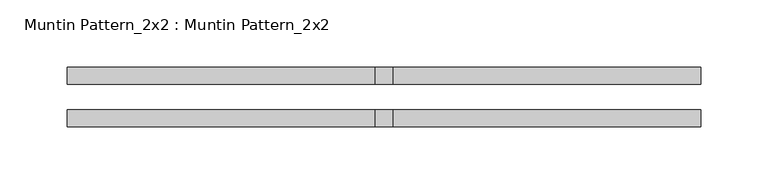
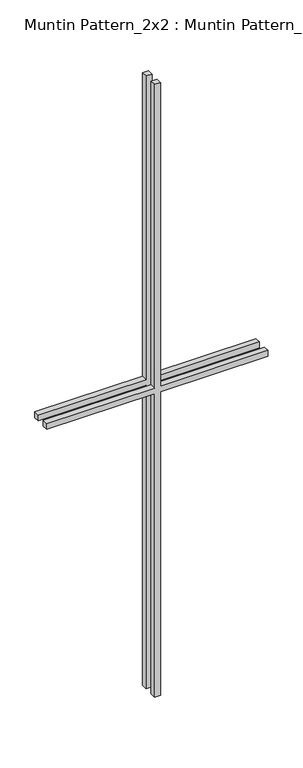
"""IFC4 building model written with IfcOpenShell, lengths in millimetres: proxy geometry, Muntin Pattern_2x2 : Muntin Pattern_2x2."""

from ifc_helpers import new_model, si_unit, frame, origin, place, context, project, spatial, polyline, outline, extrude, source, transform, mapped, element, save


def muntin_pattern_2x2_muntin_pattern_2x2_a30a3345(model_context):
    return source(origin(), model_context, "Body", "SweptSolid", [
        extrude(outline(polyline([(698.5, -6.35), (698.5, -236.5375), (685.8, -236.5375), (685.8, -6.35), (0.0, -6.35), (0.0, 6.35), (685.8, 6.35), (685.8, 236.5375), (698.5, 236.5375), (698.5, 6.35), (1384.3, 6.35), (1384.3, -6.35), (698.5, -6.35)])), frame((0.0, -22.225, 0.0), z_axis=(0.0, 1.0, 0.0), x_axis=(0.0, 0.0, 1.0)), (0.0, 0.0, 1.0), 12.7),
        extrude(outline(polyline([(698.5, -6.35), (698.5, -236.5375), (685.8, -236.5375), (685.8, -6.35), (0.0, -6.35), (0.0, 6.35), (685.8, 6.35), (685.8, 236.5375), (698.5, 236.5375), (698.5, 6.35), (1384.3, 6.35), (1384.3, -6.35), (698.5, -6.35)])), frame((0.0, 9.525, 0.0), z_axis=(0.0, 1.0, 0.0), x_axis=(0.0, 0.0, 1.0)), (0.0, 0.0, 1.0), 12.7),
    ])


if __name__ == "__main__":
    model = new_model("IFC4")
    model_context = context("Model", 3, world=origin())
    ifc_project = project(units=[si_unit("LENGTHUNIT", "METRE", prefix="MILLI")], contexts=[model_context])
    site = spatial("IfcSite", under=ifc_project)
    building = spatial("IfcBuilding", under=site)
    placement = place(None, origin())
    muntin_pattern_2x2_muntin_pattern_2x2_shape = muntin_pattern_2x2_muntin_pattern_2x2_a30a3345(model_context)
    element("IfcBuildingElementProxy", 1, Name="Muntin Pattern_2x2 : Muntin Pattern_2x2", ObjectType="Muntin Pattern_2x2 : Muntin Pattern_2x2", at=placement, inside=building, context=model_context, shape_type="MappedRepresentation", body=[
        mapped(muntin_pattern_2x2_muntin_pattern_2x2_shape, transform((0.0, 0.0, 0.0), x_axis=(1.0, 0.0, 0.0), y_axis=(0.0, 1.0, 0.0), z_axis=(0.0, 0.0, 1.0))),
    ])
    save(model, "model.ifc")

# Revit data of these elements
# Type "Muntin Pattern_2x2 : Muntin Pattern_2x2"
#   Width [instance default] = 4' - 0"
#   Thickness = 0' - 0 1/2"
#   Height [instance default] = 4' - 0"
#   Distance = 0' - 0 3/4"
#   Interior Material [instance default] = none
#   Exterior Material [instance default] = none
#   Default Elevation = 0
# Element 1 (IfcBuildingElementProxy, "Muntin Pattern_2x2 : Muntin Pattern_2x2")
#   Width = 1' - 6 5/8"
#   Height = 4' - 6 1/2"
#   Interior Material = Wood - Stained
#   Exterior Material = BLACK MATERIAL
#   Materials on its faces: "BLACK MATERIAL", "Wood - Stained"
# Materials
#   "BLACK MATERIAL": class "Generic", colour RGB 120 120 120, transparency 0, Cost = 0
#   "Wood - Stained": class "Wood", colour RGB 224 178 126, transparency 0, Cost = 0
